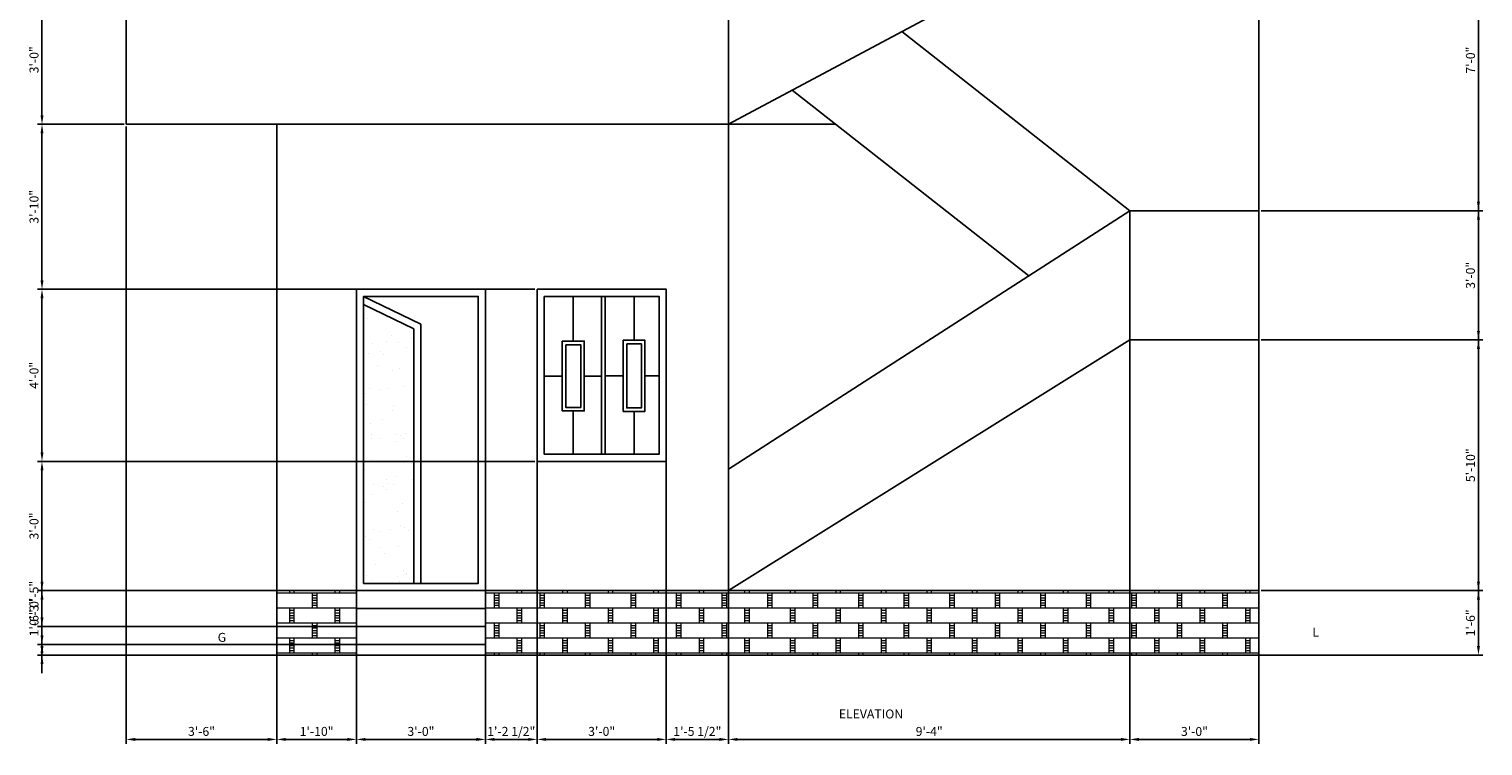
# Model space of a CAD drawing. Units: inches. Extents: x 2020 to 7901, y 1581 to 3943.
# Tile 6 of 17: x 2323 to 2729, y 2463 to 2663. Entities that reach past the tile are written whole.
import ezdxf

# ---------------------------------------------------------------- set-up
doc = ezdxf.new("R2010")
doc.units = ezdxf.units.IN
for name, color, linetype, lineweight in [('A-ANNO-DIMS', 2, 'Continuous', 18), ('A-ANNO-TEXT', 7, 'Continuous', 18), ('A-ELEV', 7, 'Continuous', 25), ('A-ELEV-PATT', 8, 'Continuous', 13)]:
    doc.layers.add(name, color=color, linetype=linetype, lineweight=lineweight)
doc.styles.get("Standard").update_dxf_attribs({"font": 'arial.ttf'})
doc.dimstyles.new('ISO-25', dxfattribs={"dimtxt": 2.5, "dimasz": 2.5, "dimexe": 1.25, "dimexo": 0.625, "dimtad": 1, "dimdec": 1, "dimlunit": 3, "dimtxsty": 'Standard', "dimcen": 2.5, "dimadec": 0, "dimazin": 0, "dimtfac": 1, "dimtdec": 1, "dimtmove": 0, "dimatfit": 3, "dimfxl": 1, "dimarcsym": 0})

# ---------------------------------------------------------------- blocks, each defined once
blk = doc.blocks.new('*D63')
at = {"layer": 'A-ANNO-DIMS', "color": 0, "lineweight": -2, "transparency": 16777216}
for p, q in [((2666.99, 2911.95), (2728.83, 2911.95)), ((2727.58, 2490.45), (2727.58, 2909.45)), ((2666.99, 2487.95), (2728.83, 2487.95))]:
    blk.add_line(p, q, dxfattribs=at)
at = {"layer": 'A-ANNO-DIMS', "color": 0, "transparency": 16777216}
for points in [[(2727.17, 2909.45), (2728, 2909.45), (2727.58, 2911.95)], [(2727.17, 2490.45), (2728, 2490.45), (2727.58, 2487.95)]]:
    blk.add_solid(points, dxfattribs=at)
at = {"layer": 'DEFPOINTS', "color": 0, "transparency": 16777216}
for p in [(2666.36, 2911.95), (2727.58, 2911.95), (2666.36, 2487.95)]:
    blk.add_point(p, dxfattribs=at)
at = {"layer": 'A-ANNO-DIMS', "color": 0, "transparency": 16777216, "insert": (2725.68, 2699.95), "char_height": 2.5, "attachment_point": 5, "rotation": 90}
blk.add_mtext('35\'-4"', dxfattribs=at)
blk = doc.blocks.new('*D64')
at = {"layer": 'A-ANNO-DIMS', "color": 0, "lineweight": -2, "transparency": 16777216}
for p, q in [((2449.94, 2505.95), (2325.61, 2505.95)), ((2326.86, 2490.45), (2326.86, 2503.45)), ((2391.74, 2487.95), (2325.61, 2487.95))]:
    blk.add_line(p, q, dxfattribs=at)
at = {"layer": 'A-ANNO-DIMS', "color": 0, "transparency": 16777216}
for points in [[(2326.45, 2503.45), (2327.28, 2503.45), (2326.86, 2505.95)], [(2326.45, 2490.45), (2327.28, 2490.45), (2326.86, 2487.95)]]:
    blk.add_solid(points, dxfattribs=at)
at = {"layer": 'DEFPOINTS', "color": 0, "transparency": 16777216}
for p in [(2326.86, 2505.95), (2450.57, 2505.95), (2392.36, 2487.95)]:
    blk.add_point(p, dxfattribs=at)
at = {"layer": 'A-ANNO-DIMS', "color": 0, "transparency": 16777216, "insert": (2324.96, 2496.95), "char_height": 2.5, "attachment_point": 5, "rotation": 90}
blk.add_mtext('1\'-6"', dxfattribs=at)
blk = doc.blocks.new('*D65')
at = {"layer": 'A-ANNO-DIMS', "color": 0, "lineweight": -2, "transparency": 16777216}
for p, q in [((2464.37, 2541.95), (2325.61, 2541.95)), ((2326.86, 2508.45), (2326.86, 2539.45)), ((2449.94, 2505.95), (2325.61, 2505.95))]:
    blk.add_line(p, q, dxfattribs=at)
at = {"layer": 'A-ANNO-DIMS', "color": 0, "transparency": 16777216}
for points in [[(2326.45, 2539.45), (2327.28, 2539.45), (2326.86, 2541.95)], [(2326.45, 2508.45), (2327.28, 2508.45), (2326.86, 2505.95)]]:
    blk.add_solid(points, dxfattribs=at)
at = {"layer": 'DEFPOINTS', "color": 0, "transparency": 16777216}
for p in [(2326.86, 2541.95), (2464.99, 2541.95), (2450.57, 2505.95)]:
    blk.add_point(p, dxfattribs=at)
at = {"layer": 'A-ANNO-DIMS', "color": 0, "transparency": 16777216, "insert": (2324.96, 2523.95), "char_height": 2.5, "attachment_point": 5, "rotation": 90}
blk.add_mtext('3\'-0"', dxfattribs=at)
blk = doc.blocks.new('*D66')
at = {"layer": 'A-ANNO-DIMS', "color": 0, "lineweight": -2, "transparency": 16777216}
for p, q in [((2464.37, 2589.95), (2325.61, 2589.95)), ((2326.86, 2544.45), (2326.86, 2587.45)), ((2464.37, 2541.95), (2325.61, 2541.95))]:
    blk.add_line(p, q, dxfattribs=at)
at = {"layer": 'A-ANNO-DIMS', "color": 0, "transparency": 16777216}
for points in [[(2326.45, 2587.45), (2327.28, 2587.45), (2326.86, 2589.95)], [(2326.45, 2544.45), (2327.28, 2544.45), (2326.86, 2541.95)]]:
    blk.add_solid(points, dxfattribs=at)
at = {"layer": 'DEFPOINTS', "color": 0, "transparency": 16777216}
for p in [(2326.86, 2589.95), (2464.99, 2589.95), (2464.99, 2541.95)]:
    blk.add_point(p, dxfattribs=at)
at = {"layer": 'A-ANNO-DIMS', "color": 0, "transparency": 16777216, "insert": (2324.96, 2565.95), "char_height": 2.5, "attachment_point": 5, "rotation": 90}
blk.add_mtext('4\'-0"', dxfattribs=at)
blk = doc.blocks.new('*D67')
at = {"layer": 'A-ANNO-DIMS', "color": 0, "lineweight": -2, "transparency": 16777216}
for p, q in [((2349.74, 2635.95), (2325.61, 2635.95)), ((2326.86, 2592.45), (2326.86, 2633.45)), ((2464.37, 2589.95), (2325.61, 2589.95))]:
    blk.add_line(p, q, dxfattribs=at)
at = {"layer": 'A-ANNO-DIMS', "color": 0, "transparency": 16777216}
for points in [[(2326.45, 2633.45), (2327.28, 2633.45), (2326.86, 2635.95)], [(2326.45, 2592.45), (2327.28, 2592.45), (2326.86, 2589.95)]]:
    blk.add_solid(points, dxfattribs=at)
at = {"layer": 'DEFPOINTS', "color": 0, "transparency": 16777216}
for p in [(2326.86, 2635.95), (2350.36, 2635.95), (2464.99, 2589.95)]:
    blk.add_point(p, dxfattribs=at)
at = {"layer": 'A-ANNO-DIMS', "color": 0, "transparency": 16777216, "insert": (2324.96, 2612.95), "char_height": 2.5, "attachment_point": 5, "rotation": 90}
blk.add_mtext('3\'-10"', dxfattribs=at)
blk = doc.blocks.new('*D68')
at = {"layer": 'A-ANNO-DIMS', "color": 0, "lineweight": -2, "transparency": 16777216}
for p, q in [((2349.74, 2671.95), (2325.61, 2671.95)), ((2326.86, 2638.45), (2326.86, 2669.45)), ((2349.74, 2635.95), (2325.61, 2635.95))]:
    blk.add_line(p, q, dxfattribs=at)
at = {"layer": 'A-ANNO-DIMS', "color": 0, "transparency": 16777216}
for points in [[(2326.45, 2669.45), (2327.28, 2669.45), (2326.86, 2671.95)], [(2326.45, 2638.45), (2327.28, 2638.45), (2326.86, 2635.95)]]:
    blk.add_solid(points, dxfattribs=at)
at = {"layer": 'DEFPOINTS', "color": 0, "transparency": 16777216}
for p in [(2326.86, 2671.95), (2350.36, 2671.95), (2350.36, 2635.95)]:
    blk.add_point(p, dxfattribs=at)
at = {"layer": 'A-ANNO-DIMS', "color": 0, "transparency": 16777216, "insert": (2324.96, 2653.95), "char_height": 2.5, "attachment_point": 5, "rotation": 90}
blk.add_mtext('3\'-0"', dxfattribs=at)
blk = doc.blocks.new('*D73')
at = {"layer": 'A-ANNO-DIMS', "color": 0, "lineweight": -2, "transparency": 16777216}
for p, q in [((2350.36, 2635.32), (2350.36, 2463.2)), ((2392.36, 2635.32), (2392.36, 2463.2)), ((2352.86, 2464.45), (2389.86, 2464.45))]:
    blk.add_line(p, q, dxfattribs=at)
at = {"layer": 'A-ANNO-DIMS', "color": 0, "transparency": 16777216}
for points in [[(2352.86, 2464.86), (2352.86, 2464.03), (2350.36, 2464.45)], [(2389.86, 2464.86), (2389.86, 2464.03), (2392.36, 2464.45)]]:
    blk.add_solid(points, dxfattribs=at)
at = {"layer": 'DEFPOINTS', "color": 0, "transparency": 16777216}
for p in [(2350.36, 2635.95), (2392.36, 2635.95), (2392.36, 2464.45)]:
    blk.add_point(p, dxfattribs=at)
at = {"layer": 'A-ANNO-DIMS', "color": 0, "transparency": 16777216, "insert": (2371.36, 2466.35), "char_height": 2.5, "attachment_point": 5}
blk.add_mtext('3\'-6"', dxfattribs=at)
blk = doc.blocks.new('*D74')
at = {"layer": 'A-ANNO-DIMS', "color": 0, "lineweight": -2, "transparency": 16777216}
for p, q in [((2392.36, 2635.32), (2392.36, 2463.2)), ((2414.57, 2589.32), (2414.57, 2463.2)), ((2394.86, 2464.45), (2412.07, 2464.45))]:
    blk.add_line(p, q, dxfattribs=at)
at = {"layer": 'A-ANNO-DIMS', "color": 0, "transparency": 16777216}
for points in [[(2394.86, 2464.86), (2394.86, 2464.03), (2392.36, 2464.45)], [(2412.07, 2464.86), (2412.07, 2464.03), (2414.57, 2464.45)]]:
    blk.add_solid(points, dxfattribs=at)
at = {"layer": 'DEFPOINTS', "color": 0, "transparency": 16777216}
for p in [(2392.36, 2635.95), (2414.57, 2589.95), (2414.57, 2464.45)]:
    blk.add_point(p, dxfattribs=at)
at = {"layer": 'A-ANNO-DIMS', "color": 0, "transparency": 16777216, "insert": (2403.47, 2466.35), "char_height": 2.5, "attachment_point": 5}
blk.add_mtext('1\'-10"', dxfattribs=at)
blk = doc.blocks.new('*D75')
at = {"layer": 'A-ANNO-DIMS', "color": 0, "lineweight": -2, "transparency": 16777216}
for p, q in [((2414.57, 2589.32), (2414.57, 2463.2)), ((2450.57, 2589.32), (2450.57, 2463.2)), ((2417.07, 2464.45), (2448.07, 2464.45))]:
    blk.add_line(p, q, dxfattribs=at)
at = {"layer": 'A-ANNO-DIMS', "color": 0, "transparency": 16777216}
for points in [[(2417.07, 2464.86), (2417.07, 2464.03), (2414.57, 2464.45)], [(2448.07, 2464.86), (2448.07, 2464.03), (2450.57, 2464.45)]]:
    blk.add_solid(points, dxfattribs=at)
at = {"layer": 'DEFPOINTS', "color": 0, "transparency": 16777216}
for p in [(2414.57, 2589.95), (2450.57, 2589.95), (2450.57, 2464.45)]:
    blk.add_point(p, dxfattribs=at)
at = {"layer": 'A-ANNO-DIMS', "color": 0, "transparency": 16777216, "insert": (2432.57, 2466.35), "char_height": 2.5, "attachment_point": 5}
blk.add_mtext('3\'-0"', dxfattribs=at)
blk = doc.blocks.new('*D76')
at = {"layer": 'A-ANNO-DIMS', "color": 0, "lineweight": -2, "transparency": 16777216}
for p, q in [((2450.57, 2589.32), (2450.57, 2463.2)), ((2464.99, 2589.32), (2464.99, 2463.2)), ((2453.07, 2464.45), (2462.49, 2464.45))]:
    blk.add_line(p, q, dxfattribs=at)
at = {"layer": 'A-ANNO-DIMS', "color": 0, "transparency": 16777216}
for points in [[(2453.07, 2464.86), (2453.07, 2464.03), (2450.57, 2464.45)], [(2462.49, 2464.86), (2462.49, 2464.03), (2464.99, 2464.45)]]:
    blk.add_solid(points, dxfattribs=at)
at = {"layer": 'DEFPOINTS', "color": 0, "transparency": 16777216}
for p in [(2450.57, 2589.95), (2464.99, 2589.95), (2464.99, 2464.45)]:
    blk.add_point(p, dxfattribs=at)
at = {"layer": 'A-ANNO-DIMS', "color": 0, "transparency": 16777216, "insert": (2457.78, 2466.36), "char_height": 2.5, "attachment_point": 5}
blk.add_mtext('1\'-2 1/2"', dxfattribs=at)
blk = doc.blocks.new('*D77')
at = {"layer": 'A-ANNO-DIMS', "color": 0, "lineweight": -2, "transparency": 16777216}
for p, q in [((2464.99, 2589.32), (2464.99, 2463.2)), ((2500.99, 2589.32), (2500.99, 2463.2)), ((2467.49, 2464.45), (2498.49, 2464.45))]:
    blk.add_line(p, q, dxfattribs=at)
at = {"layer": 'A-ANNO-DIMS', "color": 0, "transparency": 16777216}
for points in [[(2467.49, 2464.86), (2467.49, 2464.03), (2464.99, 2464.45)], [(2498.49, 2464.86), (2498.49, 2464.03), (2500.99, 2464.45)]]:
    blk.add_solid(points, dxfattribs=at)
at = {"layer": 'DEFPOINTS', "color": 0, "transparency": 16777216}
for p in [(2464.99, 2589.95), (2500.99, 2589.95), (2500.99, 2464.45)]:
    blk.add_point(p, dxfattribs=at)
at = {"layer": 'A-ANNO-DIMS', "color": 0, "transparency": 16777216, "insert": (2482.99, 2466.35), "char_height": 2.5, "attachment_point": 5}
blk.add_mtext('3\'-0"', dxfattribs=at)
blk = doc.blocks.new('*D78')
at = {"layer": 'A-ANNO-DIMS', "color": 0, "lineweight": -2, "transparency": 16777216}
for p, q in [((2518.36, 2635.32), (2518.36, 2463.2)), ((2500.99, 2589.32), (2500.99, 2463.2)), ((2503.49, 2464.45), (2515.86, 2464.45))]:
    blk.add_line(p, q, dxfattribs=at)
at = {"layer": 'A-ANNO-DIMS', "color": 0, "transparency": 16777216}
for points in [[(2503.49, 2464.86), (2503.49, 2464.03), (2500.99, 2464.45)], [(2515.86, 2464.86), (2515.86, 2464.03), (2518.36, 2464.45)]]:
    blk.add_solid(points, dxfattribs=at)
at = {"layer": 'DEFPOINTS', "color": 0, "transparency": 16777216}
for p in [(2518.36, 2635.95), (2500.99, 2589.95), (2518.36, 2464.45)]:
    blk.add_point(p, dxfattribs=at)
at = {"layer": 'A-ANNO-DIMS', "color": 0, "transparency": 16777216, "insert": (2509.68, 2466.36), "char_height": 2.5, "attachment_point": 5}
blk.add_mtext('1\'-5 1/2"', dxfattribs=at)
blk = doc.blocks.new('*D79')
at = {"layer": 'A-ANNO-DIMS', "color": 0, "lineweight": -2, "transparency": 16777216}
for p, q in [((2518.36, 2635.32), (2518.36, 2463.2)), ((2630.36, 2611.22), (2630.36, 2463.2)), ((2520.86, 2464.45), (2627.86, 2464.45))]:
    blk.add_line(p, q, dxfattribs=at)
at = {"layer": 'A-ANNO-DIMS', "color": 0, "transparency": 16777216}
for points in [[(2520.86, 2464.86), (2520.86, 2464.03), (2518.36, 2464.45)], [(2627.86, 2464.86), (2627.86, 2464.03), (2630.36, 2464.45)]]:
    blk.add_solid(points, dxfattribs=at)
at = {"layer": 'DEFPOINTS', "color": 0, "transparency": 16777216}
for p in [(2518.36, 2635.95), (2630.36, 2611.85), (2630.36, 2464.45)]:
    blk.add_point(p, dxfattribs=at)
at = {"layer": 'A-ANNO-DIMS', "color": 0, "transparency": 16777216, "insert": (2574.36, 2466.35), "char_height": 2.5, "attachment_point": 5}
blk.add_mtext('9\'-4"', dxfattribs=at)
blk = doc.blocks.new('*D80')
at = {"layer": 'A-ANNO-DIMS', "color": 0, "lineweight": -2, "transparency": 16777216}
for p, q in [((2630.36, 2611.22), (2630.36, 2463.2)), ((2666.36, 2611.22), (2666.36, 2463.2)), ((2632.86, 2464.45), (2663.86, 2464.45))]:
    blk.add_line(p, q, dxfattribs=at)
at = {"layer": 'A-ANNO-DIMS', "color": 0, "transparency": 16777216}
for points in [[(2632.86, 2464.86), (2632.86, 2464.03), (2630.36, 2464.45)], [(2663.86, 2464.86), (2663.86, 2464.03), (2666.36, 2464.45)]]:
    blk.add_solid(points, dxfattribs=at)
at = {"layer": 'DEFPOINTS', "color": 0, "transparency": 16777216}
for p in [(2630.36, 2611.85), (2666.36, 2611.85), (2666.36, 2464.45)]:
    blk.add_point(p, dxfattribs=at)
at = {"layer": 'A-ANNO-DIMS', "color": 0, "transparency": 16777216, "insert": (2648.36, 2466.35), "char_height": 2.5, "attachment_point": 5}
blk.add_mtext('3\'-0"', dxfattribs=at)
blk = doc.blocks.new('*D147')
at = {"layer": 'A-ANNO-DIMS', "color": 0, "lineweight": -2, "transparency": 16777216}
for p, q in [((2666.99, 2505.95), (2728.83, 2505.95)), ((2727.58, 2490.45), (2727.58, 2503.45)), ((2666.99, 2487.95), (2728.83, 2487.95))]:
    blk.add_line(p, q, dxfattribs=at)
at = {"layer": 'A-ANNO-DIMS', "color": 0, "transparency": 16777216}
for points in [[(2727.17, 2503.45), (2728, 2503.45), (2727.58, 2505.95)], [(2727.17, 2490.45), (2728, 2490.45), (2727.58, 2487.95)]]:
    blk.add_solid(points, dxfattribs=at)
at = {"layer": 'DEFPOINTS', "color": 0, "transparency": 16777216}
for p in [(2666.36, 2505.95), (2727.58, 2505.95), (2666.36, 2487.95)]:
    blk.add_point(p, dxfattribs=at)
at = {"layer": 'A-ANNO-DIMS', "color": 0, "transparency": 16777216, "insert": (2725.68, 2496.95), "char_height": 2.5, "attachment_point": 5, "rotation": 90}
blk.add_mtext('1\'-6"', dxfattribs=at)
blk = doc.blocks.new('*D148')
at = {"layer": 'A-ANNO-DIMS', "color": 0, "lineweight": -2, "transparency": 16777216}
for p, q in [((2666.99, 2575.85), (2728.83, 2575.85)), ((2727.58, 2508.45), (2727.58, 2573.35)), ((2666.99, 2505.95), (2728.83, 2505.95))]:
    blk.add_line(p, q, dxfattribs=at)
at = {"layer": 'A-ANNO-DIMS', "color": 0, "transparency": 16777216}
for points in [[(2727.17, 2573.35), (2728, 2573.35), (2727.58, 2575.85)], [(2727.17, 2508.45), (2728, 2508.45), (2727.58, 2505.95)]]:
    blk.add_solid(points, dxfattribs=at)
at = {"layer": 'DEFPOINTS', "color": 0, "transparency": 16777216}
for p in [(2666.36, 2575.85), (2727.58, 2575.85), (2666.36, 2505.95)]:
    blk.add_point(p, dxfattribs=at)
at = {"layer": 'A-ANNO-DIMS', "color": 0, "transparency": 16777216, "insert": (2725.68, 2540.9), "char_height": 2.5, "attachment_point": 5, "rotation": 90}
blk.add_mtext('5\'-10"', dxfattribs=at)
blk = doc.blocks.new('*D149')
at = {"layer": 'A-ANNO-DIMS', "color": 0, "lineweight": -2, "transparency": 16777216}
for p, q in [((2666.99, 2611.85), (2728.83, 2611.85)), ((2727.58, 2578.35), (2727.58, 2609.35)), ((2666.99, 2575.85), (2728.83, 2575.85))]:
    blk.add_line(p, q, dxfattribs=at)
at = {"layer": 'A-ANNO-DIMS', "color": 0, "transparency": 16777216}
for points in [[(2727.17, 2609.35), (2728, 2609.35), (2727.58, 2611.85)], [(2727.17, 2578.35), (2728, 2578.35), (2727.58, 2575.85)]]:
    blk.add_solid(points, dxfattribs=at)
at = {"layer": 'DEFPOINTS', "color": 0, "transparency": 16777216}
for p in [(2666.36, 2611.85), (2727.58, 2611.85), (2666.36, 2575.85)]:
    blk.add_point(p, dxfattribs=at)
at = {"layer": 'A-ANNO-DIMS', "color": 0, "transparency": 16777216, "insert": (2725.68, 2593.85), "char_height": 2.5, "attachment_point": 5, "rotation": 90}
blk.add_mtext('3\'-0"', dxfattribs=at)
blk = doc.blocks.new('*D150')
at = {"layer": 'A-ANNO-DIMS', "color": 0, "lineweight": -2, "transparency": 16777216}
for p, q in [((2666.99, 2695.85), (2728.83, 2695.85)), ((2727.58, 2614.35), (2727.58, 2693.35)), ((2666.99, 2611.85), (2728.83, 2611.85))]:
    blk.add_line(p, q, dxfattribs=at)
at = {"layer": 'A-ANNO-DIMS', "color": 0, "transparency": 16777216}
for points in [[(2727.17, 2693.35), (2728, 2693.35), (2727.58, 2695.85)], [(2727.17, 2614.35), (2728, 2614.35), (2727.58, 2611.85)]]:
    blk.add_solid(points, dxfattribs=at)
at = {"layer": 'DEFPOINTS', "color": 0, "transparency": 16777216}
for p in [(2666.36, 2695.85), (2727.58, 2695.85), (2666.36, 2611.85)]:
    blk.add_point(p, dxfattribs=at)
at = {"layer": 'A-ANNO-DIMS', "color": 0, "transparency": 16777216, "insert": (2725.68, 2653.85), "char_height": 2.5, "attachment_point": 5, "rotation": 90}
blk.add_mtext('7\'-0"', dxfattribs=at)
blk = doc.blocks.new('*D156')
at = {"layer": 'A-ANNO-DIMS', "color": 0, "lineweight": -2, "transparency": 16777216}
for p, q in [((2326.86, 2493.45), (2326.86, 2503.84)), ((2449.94, 2490.95), (2325.61, 2490.95)), ((2326.86, 2487.95), (2326.86, 2490.95)), ((2449.94, 2487.95), (2325.61, 2487.95)), ((2326.86, 2485.45), (2326.86, 2482.95))]:
    blk.add_line(p, q, dxfattribs=at)
at = {"layer": 'A-ANNO-DIMS', "color": 0, "transparency": 16777216}
for points in [[(2326.45, 2493.45), (2327.28, 2493.45), (2326.86, 2490.95)], [(2326.45, 2485.45), (2327.28, 2485.45), (2326.86, 2487.95)]]:
    blk.add_solid(points, dxfattribs=at)
at = {"layer": 'DEFPOINTS', "color": 0, "transparency": 16777216}
for p in [(2326.86, 2490.95), (2450.57, 2490.95), (2450.57, 2487.95)]:
    blk.add_point(p, dxfattribs=at)
at = {"layer": 'A-ANNO-DIMS', "color": 0, "transparency": 16777216, "insert": (2324.96, 2499.89), "char_height": 2.5, "attachment_point": 5, "rotation": 90}
blk.add_mtext('0\'-3"', dxfattribs=at)
blk = doc.blocks.new('*D157')
at = {"layer": 'A-ANNO-DIMS', "color": 0, "lineweight": -2, "transparency": 16777216}
for p, q in [((2326.86, 2498.45), (2326.86, 2508.84)), ((2449.94, 2495.95), (2325.61, 2495.95)), ((2326.86, 2490.95), (2326.86, 2495.95)), ((2449.94, 2490.95), (2325.61, 2490.95)), ((2326.86, 2488.45), (2326.86, 2485.95))]:
    blk.add_line(p, q, dxfattribs=at)
at = {"layer": 'A-ANNO-DIMS', "color": 0, "transparency": 16777216}
for points in [[(2326.45, 2498.45), (2327.28, 2498.45), (2326.86, 2495.95)], [(2326.45, 2488.45), (2327.28, 2488.45), (2326.86, 2490.95)]]:
    blk.add_solid(points, dxfattribs=at)
at = {"layer": 'DEFPOINTS', "color": 0, "transparency": 16777216}
for p in [(2326.86, 2495.95), (2450.57, 2495.95), (2450.57, 2490.95)]:
    blk.add_point(p, dxfattribs=at)
at = {"layer": 'A-ANNO-DIMS', "color": 0, "transparency": 16777216, "insert": (2324.96, 2504.89), "char_height": 2.5, "attachment_point": 5, "rotation": 90}
blk.add_mtext('0\'-5"', dxfattribs=at)

msp = doc.modelspace()

# ---------------------------------------------------------------- hatches: boundary and pattern name
at = {"layer": 'A-ELEV-PATT'}
h = msp.add_hatch(dxfattribs=at)
h.set_pattern_fill('AR-SAND', color=256, scale=0.2)
h.set_pattern_definition([(37.5, (-52.601, -26.04), (-0.320006, 9.788265), [0, -7.7216, 0, -8.636, 0, -8.255]), (7.5, (-52.601, -26.04), (8.990466, 14.3365), [0, -4.1656, 0, -6.9596, 0, -2.667]), (327.5, (-58.849, -26.04), (15.819847, 0.028744), [0, -2.54, 0, -9.144, 0, -11.938]), (317.5, (-58.85, -26.04), (15.27113, 4.458586), [0, -1.27, 0, -5.9944, 0, -6.858])])
h.paths.add_polyline_path([(2430.57, 2578.94), (2416.57, 2585.72), (2416.57, 2507.95), (2430.57, 2507.95)])
h = msp.add_hatch(dxfattribs=at)
h.set_pattern_fill('BRSTONE', color=256, scale=0.5)
h.set_pattern_definition([(0, (-52.601, -26.04), (0, 4.191), []), (90, (-41.171, -26.04), (-6.35, 4.191), [4.191, -4.191]), (90, (-42.441, -26.04), (-6.35, 4.191), [4.191, -4.191]), (0, (-41.171, -25.3414), (6.35, 4.191), [-11.43, 1.27]), (0, (-41.171, -24.643), (6.35, 4.191), [-11.43, 1.27]), (0, (-41.171, -23.9444), (6.35, 4.191), [-11.43, 1.27]), (0, (-41.171, -23.246), (6.35, 4.191), [-11.43, 1.27]), (0, (-41.171, -22.5474), (6.35, 4.191), [-11.43, 1.27])])
h.paths.add_polyline_path([(2666.36, 2505.95), (2450.57, 2505.95), (2450.57, 2487.95), (2666.36, 2487.95)])
h.paths.add_polyline_path([(2414.57, 2505.95), (2392.36, 2505.95), (2392.36, 2487.95), (2414.57, 2487.95)])

# ---------------------------------------------------------------- linework, layer by layer
at = {"layer": 'A-ELEV'}
for p, q in [((2666.36, 2487.95), (2666.36, 2911.95)), ((2518.36, 2635.95), (2630.36, 2695.85)), ((2350.36, 2635.95), (2350.36, 2671.95)), ((2518.36, 2505.95), (2518.36, 2671.95)), ((2630.36, 2611.85), (2566.69, 2661.79)), ((2602.14, 2593.69), (2536.15, 2645.46)), ((2392.36, 2635.95), (2350.36, 2635.95)), ((2392.36, 2487.95), (2392.36, 2635.95)), ((2548.27, 2635.95), (2392.36, 2635.95)), ((2630.36, 2611.85), (2518.36, 2539.81)), ((2666.36, 2611.85), (2630.36, 2611.85)), ((2630.36, 2611.85), (2630.36, 2575.85)), ((2416.57, 2587.95), (2432.57, 2580.2)), ((2475.07, 2575.51), (2475.07, 2587.95)), ((2482.99, 2587.95), (2482.99, 2543.95)), ((2483.99, 2587.95), (2483.99, 2543.95)), ((2492.02, 2575.74), (2492.02, 2587.95)), ((2416.57, 2585.72), (2430.57, 2578.94)), ((2432.57, 2580.2), (2432.57, 2507.95)), ((2430.57, 2578.94), (2430.57, 2507.95)), ((2518.36, 2505.95), (2630.36, 2575.85)), ((2630.36, 2575.85), (2666.36, 2575.85)), ((2471.99, 2565.77), (2466.99, 2565.77)), ((2478.15, 2565.77), (2482.99, 2565.77)), ((2488.99, 2565.82), (2483.99, 2565.82)), ((2495.06, 2565.82), (2498.99, 2565.82)), ((2475.07, 2556.02), (2475.07, 2543.95)), ((2492.02, 2555.9), (2492.02, 2543.95)), ((2666.36, 2505.95), (2392.36, 2505.95)), ((2414.57, 2505.95), (2414.57, 2487.95)), ((2450.57, 2505.95), (2450.57, 2487.95)), ((2414.57, 2500.95), (2450.57, 2500.95)), ((2414.57, 2495.95), (2450.57, 2495.95)), ((2414.57, 2490.95), (2450.57, 2490.95)), ((2392.36, 2487.95), (2360.46, 2487.95)), ((2666.36, 2487.95), (2392.36, 2487.95)), ((2666.36, 2487.95), (2704.08, 2487.95))]:
    msp.add_line(p, q, dxfattribs=at)
for points in [[(2414.57, 2505.95), (2450.57, 2505.95), (2450.57, 2589.95), (2414.57, 2589.95)], [(2416.57, 2507.95), (2448.57, 2507.95), (2448.57, 2587.95), (2416.57, 2587.95)], [(2464.99, 2589.95), (2500.99, 2589.95), (2500.99, 2541.95), (2464.99, 2541.95)], [(2466.99, 2587.95), (2498.99, 2587.95), (2498.99, 2543.95), (2466.99, 2543.95)], [(2471.99, 2575.51), (2478.15, 2575.51), (2478.15, 2556.02), (2471.99, 2556.02)], [(2488.99, 2575.74), (2495.06, 2575.74), (2495.06, 2555.9), (2488.99, 2555.9)], [(2472.99, 2574.51), (2477.15, 2574.51), (2477.15, 2557.02), (2472.99, 2557.02)], [(2489.99, 2574.74), (2494.06, 2574.74), (2494.06, 2556.9), (2489.99, 2556.9)]]:
    msp.add_lwpolyline(points, close=True, dxfattribs=at)

# ---------------------------------------------------------------- texts
at = {"layer": 'A-ANNO-TEXT', "char_height": 2.5, "attachment_point": 1}
for s, width, insert in [('L', 13.9246, (2681.27, 2495.58)), ('G', 10.1909, (2375.87, 2494.15)), ('ELEVATION', 132.5884, (2549.15, 2472.79))]:
    msp.add_mtext_dynamic_manual_height_columns(s, width=width, gutter_width=12.5, heights=[0], dxfattribs=dict(at, insert=insert))

# ---------------------------------------------------------------- dimensions: what is measured, and where the dimension line sits
at = {"layer": 'A-ANNO-DIMS'}
for base, p1, p2, picture, middle in [((2727.58, 2911.95), (2666.36, 2487.95), (2666.36, 2911.95), '*D63', (2725.68, 2699.95)), ((2727.58, 2695.85), (2666.36, 2611.85), (2666.36, 2695.85), '*D150', (2725.68, 2653.85)), ((2326.86, 2671.95), (2350.36, 2635.95), (2350.36, 2671.95), '*D68', (2324.96, 2653.95)), ((2326.86, 2635.95), (2464.99, 2589.95), (2350.36, 2635.95), '*D67', (2324.96, 2612.95)), ((2727.58, 2611.85), (2666.36, 2575.85), (2666.36, 2611.85), '*D149', (2725.68, 2593.85)), ((2326.86, 2589.95), (2464.99, 2541.95), (2464.99, 2589.95), '*D66', (2324.96, 2565.95)), ((2727.58, 2575.85), (2666.36, 2505.95), (2666.36, 2575.85), '*D148', (2725.68, 2540.9)), ((2326.86, 2541.95), (2450.57, 2505.95), (2464.99, 2541.95), '*D65', (2324.96, 2523.95)), ((2326.86, 2495.95), (2450.57, 2490.95), (2450.57, 2495.95), '*D157', (2324.96, 2504.89)), ((2326.86, 2505.95), (2392.36, 2487.95), (2450.57, 2505.95), '*D64', (2324.96, 2496.95)), ((2326.86, 2490.95), (2450.57, 2487.95), (2450.57, 2490.95), '*D156', (2324.96, 2499.89)), ((2727.58, 2505.95), (2666.36, 2487.95), (2666.36, 2505.95), '*D147', (2725.68, 2496.95))]:
    dim = msp.add_linear_dim(base=base, p1=p1, p2=p2, angle=90, dimstyle='ISO-25', override={"dimdec": 1, "dimlfac": 1, "dimrnd": 0, "dimzin": 1, "dimdsep": 46, "dimlunit": 4, "dimfrac": 2}, dxfattribs=at)
    dim.commit()
    dim.dimension.update_dxf_attribs({"geometry": picture, "text_midpoint": middle})
for base, p1, p2, picture, middle in [((2392.36, 2464.45), (2350.36, 2635.95), (2392.36, 2635.95), '*D73', (2371.36, 2466.35)), ((2414.57, 2464.45), (2392.36, 2635.95), (2414.57, 2589.95), '*D74', (2403.47, 2466.35)), ((2518.36, 2464.45), (2500.99, 2589.95), (2518.36, 2635.95), '*D78', (2509.68, 2466.36)), ((2630.36, 2464.45), (2518.36, 2635.95), (2630.36, 2611.85), '*D79', (2574.36, 2466.35)), ((2666.36, 2464.45), (2630.36, 2611.85), (2666.36, 2611.85), '*D80', (2648.36, 2466.35)), ((2450.57, 2464.45), (2414.57, 2589.95), (2450.57, 2589.95), '*D75', (2432.57, 2466.35)), ((2464.99, 2464.45), (2450.57, 2589.95), (2464.99, 2589.95), '*D76', (2457.78, 2466.36)), ((2500.99, 2464.45), (2464.99, 2589.95), (2500.99, 2589.95), '*D77', (2482.99, 2466.35))]:
    dim = msp.add_linear_dim(base=base, p1=p1, p2=p2, dimstyle='ISO-25', override={"dimdec": 1, "dimlfac": 1, "dimrnd": 0, "dimzin": 1, "dimdsep": 46, "dimlunit": 4, "dimfrac": 2}, dxfattribs=at)
    dim.commit()
    dim.dimension.update_dxf_attribs({"geometry": picture, "text_midpoint": middle})

doc.saveas('drawing.dxf')
